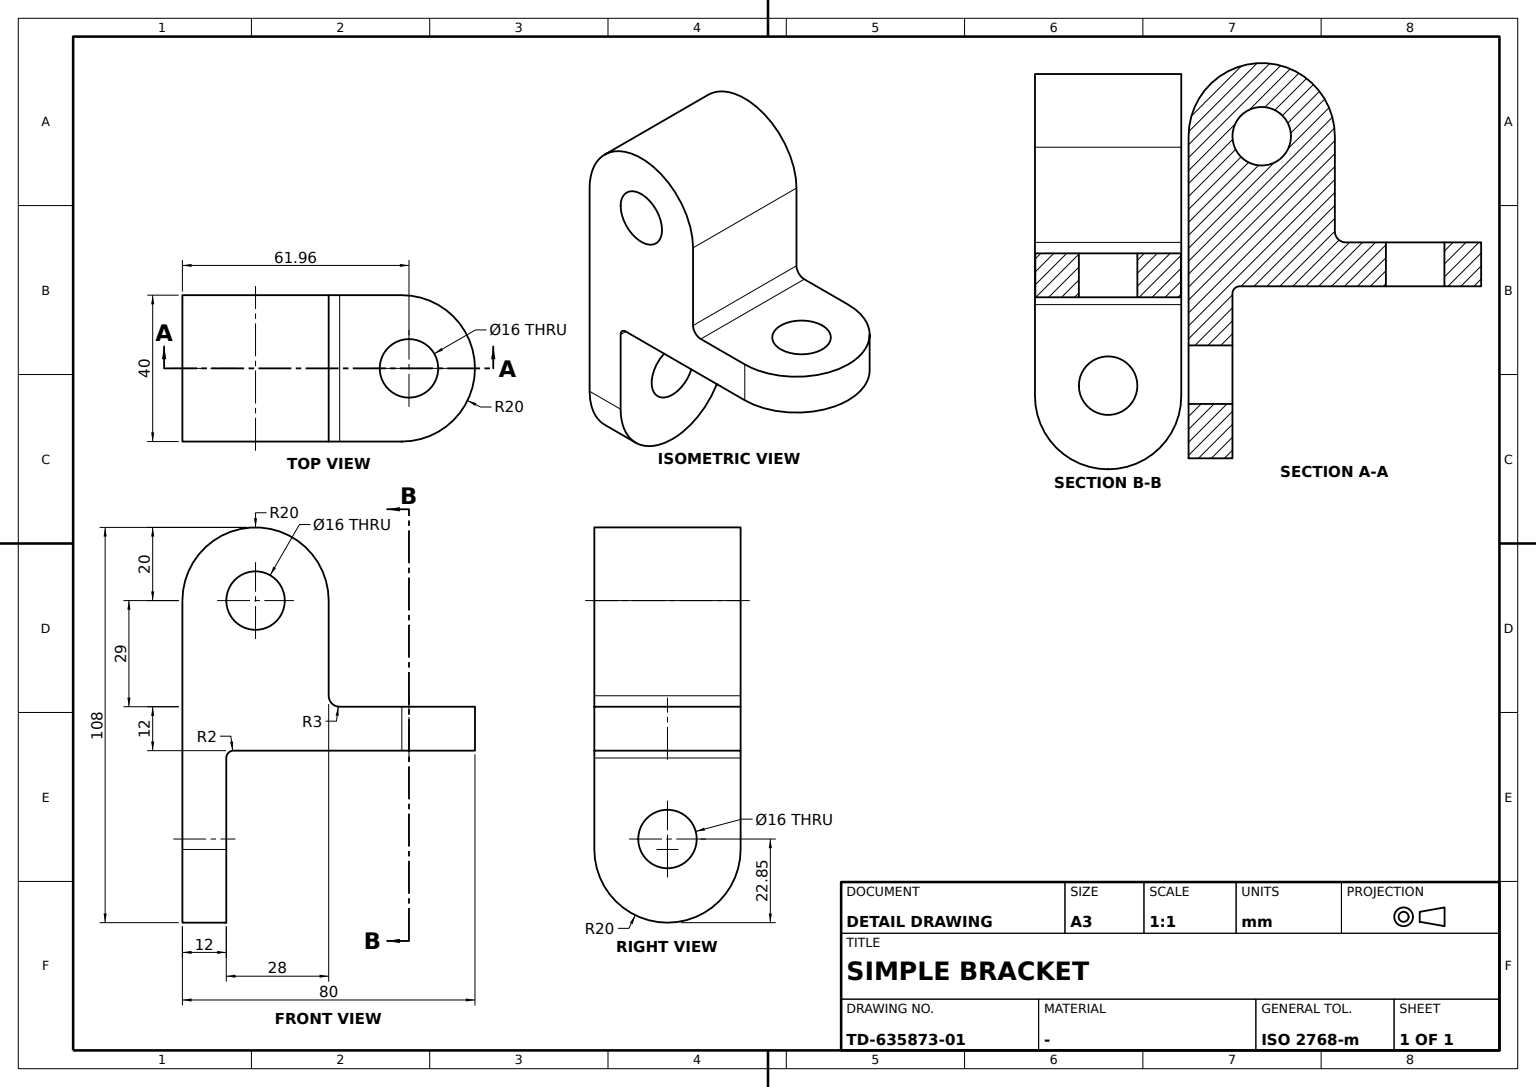
CATIA V5 part; units mm, degrees
sketch "Sketch1" plane through (0, 0, 0) normal (1, 0, 0) x (0, 1, 0)
  arc A0 (20, 0) -> (-20, 0) centre (0, 0) ccw
  circle A1 centre (0, 0) radius 8
  point P0 (-20, 0)
  line L0 (-20, 0) -> (-20, -29)
  point P1 (-20, -88)
  line L1 (-20, -88) -> (-8, -88)
  point P2 (20, 0)
  point P3 (20, 0)
  line L2 (20, 0) -> (20, -26)
  point P4 (20, -29)
  line L3 (23, -29) -> (60, -29)
  point P5 (60, -29)
  line L4 (60, -29) -> (60, -41)
  point P6 (-8, -41)
  line L5 (-8, -43) -> (-8, -88)
  line L6 (-6, -41) -> (32, -41)
  point P7 (32, -41)
  line L7 (32, -41) -> (60, -41)
  arc A2 (-6, -41) -> (-8, -43) centre (-6, -43) ccw
  line L8 (23, -29) -> (-20, -29) construction
  arc A3 (20, -26) -> (23, -29) centre (23, -26) ccw
  point P8 (20.8787, -28.1213)
  line L9 (-20, -29) -> (-20, -88)
  dimension "radius A0" = 20
  dimension "radius A1" = 8
  dimension "length L1" = 12
  dimension "length L4" = 12
  dimension "distance P6 P7" = 40
  dimension "radius A2" = 2
  dimension "distance L0 L4" = 80
  dimension "distance P3 P4" = 29
  dimension "distance P4 P5" = 40
  dimension "radius A3" = 3
  dimension "distance P0 P1" = 88
  constraint coincidence P0 x-axis
  constraint coincidence P2 A0
  constraint coincidence P2 x-axis
  constraint coincidence L6 P6
  constraint coincidence L5 P6
  constraint coincidence L2 P4
  constraint coincidence L3 P4
  constraint coincidence P4 L8
  constraint coincidence L0 L9
  constraint tangency L0 A0
  constraint tangency L2 A0
  constraint tangency A2 L6
  constraint tangency A2 L5
  constraint tangency A3 L2
  constraint tangency A3 L3
  constraint horizontal L1 x-axis
  constraint horizontal L3 x-axis
  constraint horizontal L6 x-axis
  constraint horizontal L7 x-axis
  constraint horizontal L8 x-axis
  constraint vertical L4 y-axis
  constraint vertical L5 y-axis
extrude "Pad1" add sketch "Sketch1" along normal mid plane 40
fillet "Fillet1" radius 20 2 edges at (20, 60, -35) (-20, 60, -35)
fillet "Fillet2" radius 20 2 edges at (20, -14, -88) (-20, -14, -88)
sketch "Sketch2" plane through (0, 0, -29) normal (0, 0, 1) x (1, 0, 0)
  circle A0 centre (0, 41.9556) radius 8
  point P0 (0, 41.9556)
  dimension "radius A0" = 8
  dimension "D2" = 18.0444
  constraint coincidence P0 y-axis
extrude "Pocket1" cut sketch "Sketch2" against normal up to next
sketch "Sketch3" plane through (0, -8, 0) normal (0, 1, 0) x (-1, 0, 0)
  circle A0 centre (0, -65.1459) radius 8
  point P0 (0, -65.1459)
  dimension "radius A0" = 8
  constraint coincidence P0 y-axis
extrude "Pocket2" cut sketch "Sketch3" against normal up to next
properties part number "U-Shaped Fork Bracket with Rounded Mounting Holes"
